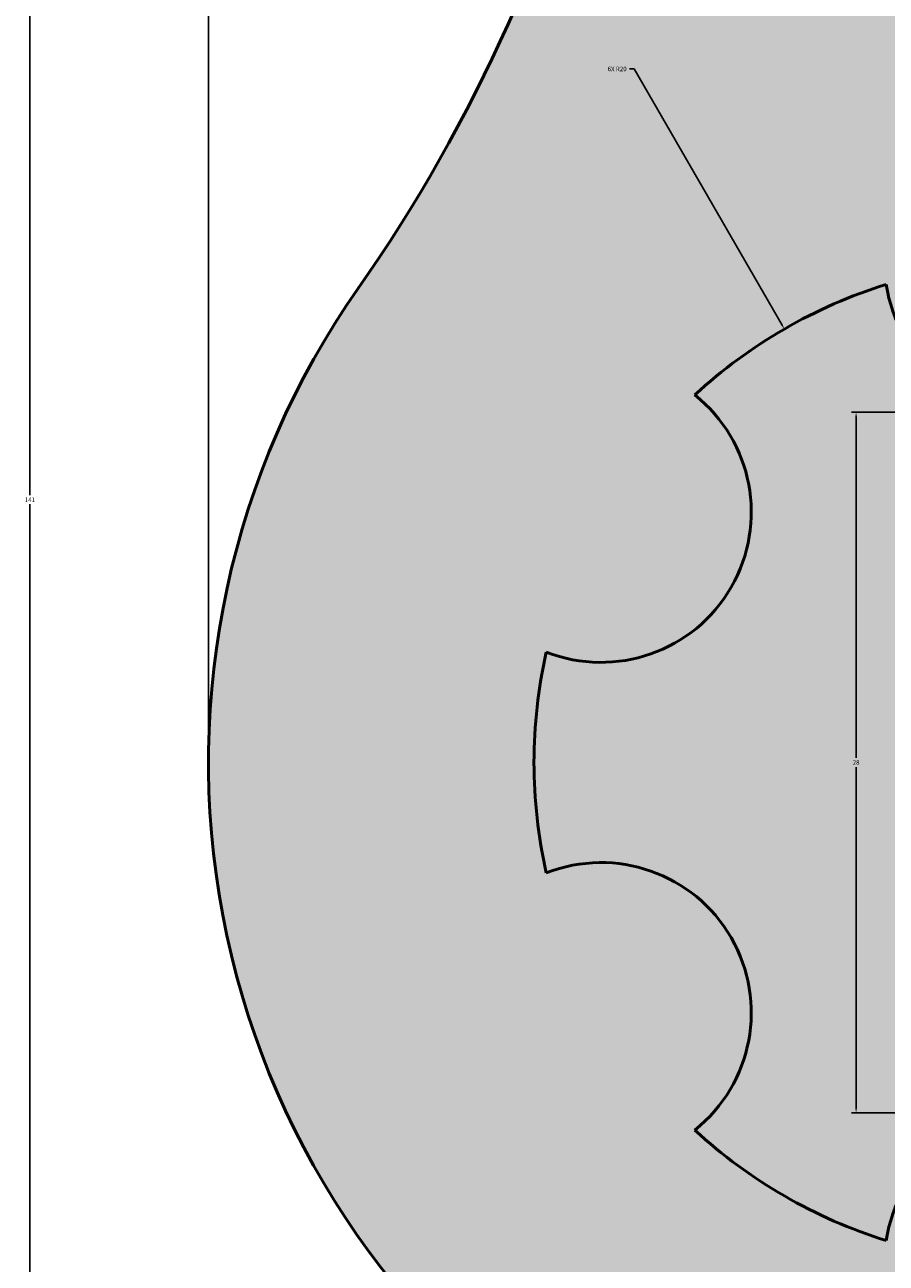
# Model space of a CAD drawing. Units: inches. Extents: x -13 to 107, y -48 to 102.
# Tile 5 of 13: x -13 to 22, y -7 to 43. Entities that reach past the tile are written whole.
import ezdxf

# ---------------------------------------------------------------- set-up
doc = ezdxf.new("R2010")
doc.units = ezdxf.units.IN
doc.header["$MEASUREMENT"] = 0
for name, color, linetype, lineweight in [('M-DIMS', 2, 'Continuous', 18), ('M-HATC', 8, 'Continuous', 18), ('M-OUTL', 7, 'Continuous', 50)]:
    doc.layers.add(name, color=color, linetype=linetype, lineweight=lineweight)
doc.styles.get("Standard").update_dxf_attribs({"font": 'arial.ttf'})
doc.dimstyles.get("Standard").update_dxf_attribs({"dimtxt": 0.18, "dimasz": 0.18, "dimexe": 0.18, "dimexo": 0.0625, "dimgap": 0.09, "dimtad": 0, "dimtih": 1, "dimtoh": 1, "dimdec": 4, "dimzin": 0, "dimdsep": 46, "dimtxsty": 'Standard', "dimcen": 0.09, "dimadec": 0, "dimazin": 0, "dimtfac": 1, "dimtdec": 4, "dimtofl": 0, "dimtmove": 0, "dimatfit": 3, "dimfxl": 1, "dimtolj": 1, "dimtzin": 0, "dimarcsym": 0})

# ---------------------------------------------------------------- blocks, each defined once
blk = doc.blocks.new('*D1')
at = {"layer": 'Defpoints', "color": 0, "transparency": 16777216}
for p in [(60.544, 101.543), (-5.45, 13.883), (60.544, 13.883)]:
    blk.add_point(p, dxfattribs=at)
at = {"layer": 'M-DIMS', "color": 0, "lineweight": -2, "transparency": 16777216}
for p, q in [((-5.45, 13.945), (-5.45, 101.723)), ((-5.27, 101.543), (27.328, 101.543)), ((60.364, 101.543), (27.766, 101.543)), ((60.544, 13.945), (60.544, 101.723))]:
    blk.add_line(p, q, dxfattribs=at)
at = {"layer": 'M-DIMS', "color": 0, "transparency": 16777216}
for points in [[(-5.27, 101.573), (-5.27, 101.513), (-5.45, 101.543)], [(60.364, 101.573), (60.364, 101.513), (60.544, 101.543)]]:
    blk.add_solid(points, dxfattribs=at)
at = {"layer": 'M-DIMS', "color": 0, "transparency": 16777216, "insert": (27.547, 101.543), "char_height": 0.18, "attachment_point": 5}
blk.add_mtext('\\A1;66', dxfattribs=at)
blk = doc.blocks.new('*D2')
at = {"layer": 'Defpoints', "color": 0, "transparency": 16777216}
for p in [(-12.585, 94.408), (27.547, 94.408), (27.547, -46.592)]:
    blk.add_point(p, dxfattribs=at)
at = {"layer": 'M-DIMS', "color": 0, "lineweight": -2, "transparency": 16777216}
for p, q in [((27.484, 94.408), (-12.765, 94.408)), ((-12.585, 94.228), (-12.585, 24.088)), ((-12.585, -46.412), (-12.585, 23.727)), ((27.484, -46.592), (-12.765, -46.592))]:
    blk.add_line(p, q, dxfattribs=at)
at = {"layer": 'M-DIMS', "color": 0, "transparency": 16777216}
for points in [[(-12.615, 94.228), (-12.555, 94.228), (-12.585, 94.408)], [(-12.615, -46.412), (-12.555, -46.412), (-12.585, -46.592)]]:
    blk.add_solid(points, dxfattribs=at)
at = {"layer": 'M-DIMS', "color": 0, "transparency": 16777216, "insert": (-12.585, 23.908), "char_height": 0.18, "attachment_point": 5}
blk.add_mtext('\\A1;141', dxfattribs=at)
blk = doc.blocks.new('*D5')
at = {"layer": 'Defpoints', "color": 0, "transparency": 16777216}
for p in [(20.412, 27.408), (27.547, 27.408), (27.547, -0.592)]:
    blk.add_point(p, dxfattribs=at)
at = {"layer": 'M-DIMS', "color": 0, "lineweight": -2, "transparency": 16777216}
for p, q in [((27.484, 27.408), (20.232, 27.408)), ((20.412, 27.228), (20.412, 13.59)), ((20.412, -0.412), (20.412, 13.226)), ((27.484, -0.592), (20.232, -0.592))]:
    blk.add_line(p, q, dxfattribs=at)
at = {"layer": 'M-DIMS', "color": 0, "transparency": 16777216}
for points in [[(20.382, 27.228), (20.442, 27.228), (20.412, 27.408)], [(20.382, -0.412), (20.442, -0.412), (20.412, -0.592)]]:
    blk.add_solid(points, dxfattribs=at)
at = {"layer": 'M-DIMS', "color": 0, "transparency": 16777216, "insert": (20.412, 13.408), "char_height": 0.18, "attachment_point": 5}
blk.add_mtext('\\A1;28', dxfattribs=at)
blk = doc.blocks.new('*D9')
at = {"layer": 'Defpoints', "color": 0, "transparency": 16777216}
for p in [(17.547, 30.728), (27.547, 13.408)]:
    blk.add_point(p, dxfattribs=at)
at = {"layer": 'M-DIMS', "color": 0, "lineweight": -2, "transparency": 16777216}
for p, q in [((11.367, 41.121), (11.547, 41.121)), ((11.547, 41.121), (17.457, 30.884)), ((27.457, 13.408), (27.637, 13.408)), ((27.547, 13.318), (27.547, 13.498))]:
    blk.add_line(p, q, dxfattribs=at)
at = {"layer": 'M-DIMS', "color": 0, "transparency": 16777216}
blk.add_solid([(17.483, 30.899), (17.431, 30.869), (17.547, 30.728)], dxfattribs=at)
at = {"layer": 'M-DIMS', "color": 0, "transparency": 16777216, "insert": (10.868, 41.121), "char_height": 0.18, "attachment_point": 5}
blk.add_mtext('\\A1;6X R20', dxfattribs=at)

msp = doc.modelspace()

# ---------------------------------------------------------------- hatches: boundary and pattern name
at = {"layer": 'M-HATC'}
h = msp.add_hatch(color=256, dxfattribs=at)
h.set_gradient(color1=(88, 186, 72), color2=(241, 235, 31), tint=1)
h.paths.add_polyline_path([(45.86, -14.044, 0.420873), (54.577, 32.339, -0.184081), (43.437, 76.537, 1.124637), (11.657, 76.537, -0.184081), (0.517, 32.339, 0.420873), (9.234, -14.044, -0.304084), (17.743, -34.622, 1.220926), (37.351, -34.622, -0.304084)])
h.paths.add_polyline_path([(33.479, -5.692, 0.859727), (21.615, -5.692, -0.111692), (13.972, -1.28, 0.859727), (8.04, 8.995, -0.111692), (8.04, 17.82, 0.859727), (13.972, 28.095, -0.111692), (21.615, 32.508, 0.859727), (33.479, 32.508, -0.111692), (41.122, 28.095, 0.859727), (47.054, 17.82, -0.111692), (47.054, 8.995, 0.859727), (41.122, -1.28, -0.111692)], flags=16)
h.paths.add_polyline_path([(32.547, -36.592, -1), (22.547, -36.592, -1)], flags=16)
h.paths.add_polyline_path([(17.547, 78.408, -1), (37.547, 78.408, -1)], flags=16)
h = msp.add_hatch(color=256, dxfattribs=at)
h.set_gradient(color1=(0, 0, 255), tint=1)
h.paths.add_polyline_path([(47.054, 8.995, 0.111692), (47.054, 17.82, -0.859727), (41.122, 28.095, 0.111692), (33.479, 32.508, -0.859727), (21.615, 32.508, 0.111692), (13.972, 28.095, -0.859727), (8.04, 17.82, 0.111692), (8.04, 8.995, -0.859727), (13.972, -1.28, 0.111692), (21.615, -5.692, -0.859727), (33.479, -5.692, 0.111692), (41.122, -1.28, -0.859727)])
h.paths.add_polyline_path([(37.547, 78.408, 1), (17.547, 78.408, 1)])
h.paths.add_polyline_path([(32.547, -36.592, 1), (22.547, -36.592, 1)])

# ---------------------------------------------------------------- linework, layer by layer
at = {"layer": 'M-OUTL'}
for centre, radius, start, end in [((-51.904, 69.054), 64, 324.99334, 8.4041), ((27.547, 13.408), 33, 144.9933, 236.293), ((27.547, 13.408), 20, 107.2539, 132.7461), ((27.547, 33.408), 6, 188.6269, 351.3731), ((10.226, 23.408), 6, 248.6269, 51.3731), ((27.547, 13.408), 20, 167.2539, 192.7461), ((10.226, 3.408), 6, 308.6269, 111.3731), ((27.547, -6.592), 6, 8.6269, 171.3731), ((27.547, 13.408), 20, 227.2539, 252.7461)]:
    msp.add_arc(centre, radius, start, end, dxfattribs=at)

# ---------------------------------------------------------------- dimensions: what is measured, and where the dimension line sits
at = {"layer": 'M-DIMS'}
dim = msp.add_linear_dim(base=(60.544, 101.543), p1=(-5.45, 13.883), p2=(60.544, 13.883), dimstyle='Standard', override={"dimdec": 0, "dimlfac": 1, "dimrnd": 0, "dimzin": 0, "dimdsep": 46, "dimlunit": 2}, dxfattribs=at)
dim.commit()
dim.dimension.update_dxf_attribs({"geometry": '*D1', "text_midpoint": (27.547, 101.543)})
for base, p1, p2, picture, middle in [((-12.585, 94.408), (27.547, -46.592), (27.547, 94.408), '*D2', (-12.585, 23.908)), ((20.412, 27.408), (27.547, -0.592), (27.547, 27.408), '*D5', (20.412, 13.408))]:
    dim = msp.add_linear_dim(base=base, p1=p1, p2=p2, angle=90, dimstyle='Standard', override={"dimdec": 0, "dimlfac": 1, "dimrnd": 0, "dimzin": 0, "dimdsep": 46, "dimlunit": 2}, dxfattribs=at)
    dim.commit()
    dim.dimension.update_dxf_attribs({"geometry": picture, "text_midpoint": middle})
dim = msp.add_radius_dim(center=(27.547, 13.408), mpoint=(17.547, 30.728), text='6X <>', dimstyle='Standard', override={"dimdec": 0, "dimlfac": 1, "dimrnd": 0, "dimzin": 0, "dimdsep": 46, "dimlunit": 2}, dxfattribs=at)
dim.commit()
dim.dimension.update_dxf_attribs({"geometry": '*D9', "text_midpoint": (10.868, 41.121), "dimtype": 164})

doc.saveas('drawing.dxf')
